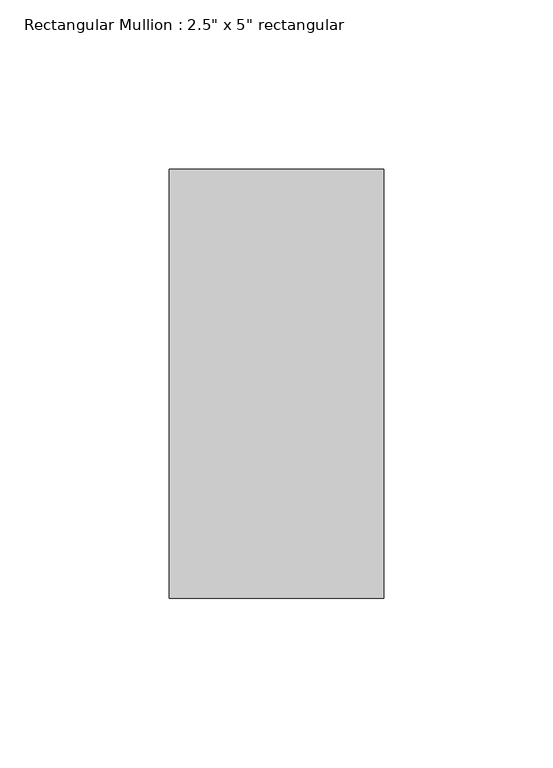
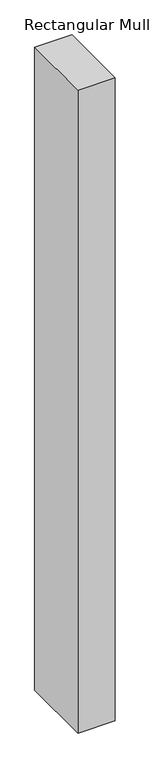
"""IFC4 building model written with IfcOpenShell, lengths in millimetres: member geometry."""

from ifc_helpers import new_model, si_unit, frame, origin, place, context, project, spatial, polyline, outline, extrude, source, transform, mapped, element, save


def member_d7472725(model_context):
    return source(origin(), model_context, "Body", "SweptSolid", [
        extrude(outline(polyline([(0.0, 63.5), (0.0, -63.5), (-63.5, -63.5), (-63.5, 63.5), (0.0, 63.5)])), frame((0.0, 0.0, -1155.7), z_axis=(0.0, 0.0, 1.0), x_axis=(1.0, 0.0, 0.0)), (0.0, 0.0, 1.0), 1155.7),
    ])


if __name__ == "__main__":
    model = new_model("IFC4")
    model_context = context("Model", 3, world=origin())
    ifc_project = project(units=[si_unit("LENGTHUNIT", "METRE", prefix="MILLI")], contexts=[model_context])
    site = spatial("IfcSite", under=ifc_project)
    building = spatial("IfcBuilding", under=site)
    placement = place(None, origin())
    member_shape = member_d7472725(model_context)
    element("IfcMember", 1, ObjectType="Rectangular Mullion : 2.5\" x 5\" rectangular", at=placement, inside=building, context=model_context, shape_type="MappedRepresentation", body=[
        mapped(member_shape, transform((0.0, 0.0, 0.0), x_axis=(1.0, 0.0, 0.0), y_axis=(0.0, 1.0, 0.0), z_axis=(0.0, 0.0, 1.0))),
    ])
    save(model, "model.ifc")

# Revit data of these elements
# Type "Rectangular Mullion : 2.5\" x 5\" rectangular"
#   built-in parameter 1007304 = 0.416667 (stored number, unit not read)
#   built-in parameter 1007301 = 0.104167 (stored number, unit not read)
#   built-in parameter 1007300 = 0.104167 (stored number, unit not read)
# Element 1 (IfcMember, "Rectangular Mullion : 2.5\" x 5\" rectangular")
#   Materials on its faces: "Aluminum"
# Materials
#   "Aluminum": class "Metal", colour RGB 247 247 247, transparency 0, Description = "Aluminum 6061", Cost = 0
